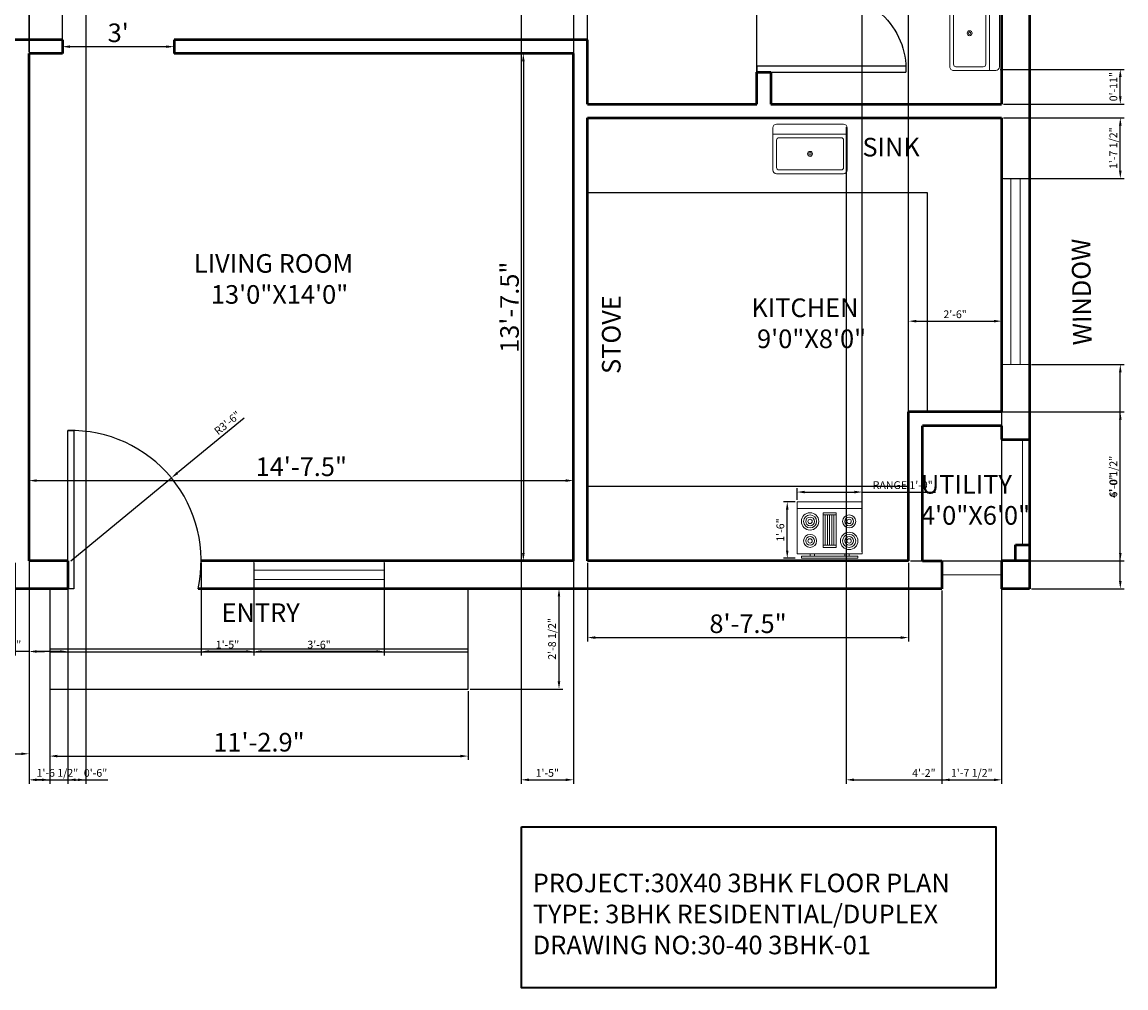
# Model space of a CAD drawing. Units: inches. Extents: x 259417 to 260009, y 246275 to 246915.
# Tile 2 of 4: x 259653 to 260009, y 246275 to 246587. Entities that reach past the tile are written whole.
import ezdxf

# ---------------------------------------------------------------- set-up
doc = ezdxf.new("R2010")
doc.units = ezdxf.units.IN
for name, color, linetype, lineweight in [('A-ANNO-DIMS', 2, 'Continuous', 18), ('A-ANNO-TEXT', 7, 'Continuous', 18), ('A-ANNO-TTLB', 7, 'Continuous', 35), ('A-AREA-IDEN', 7, 'Continuous', 25), ('A-DOOR', 3, 'Continuous', 25), ('A-EQPM', 9, 'Continuous', 18), ('A-FLOR-CASE', 9, 'Continuous', 25), ('A-FLOR-FIXT', 8, 'Continuous', 18), ('A-FLOR-STRS', 7, 'Continuous', 25), ('A-GLAZ', 4, 'Continuous', 18), ('A-WALL', 7, 'Continuous', 50)]:
    doc.layers.add(name, color=color, linetype=linetype, lineweight=lineweight)
doc.styles.get("Standard").update_dxf_attribs({"font": 'arial.ttf'})
doc.dimstyles.new('ISO-25', dxfattribs={"dimtxt": 2.5, "dimasz": 2.5, "dimexe": 1.25, "dimexo": 0.625, "dimtad": 1, "dimdec": 1, "dimlunit": 3, "dimtxsty": 'Standard', "dimcen": 2.5, "dimadec": 0, "dimazin": 0, "dimtfac": 1, "dimtdec": 1, "dimtmove": 0, "dimatfit": 3, "dimfxl": 1, "dimarcsym": 0})

# ---------------------------------------------------------------- blocks, each defined once
blk = doc.blocks.new('*D15')
at = {"layer": 'A-ANNO-DIMS', "color": 0, "lineweight": -2, "transparency": 16777216}
for p, q in [((259655.09, 246413.47), (259655.09, 246439.94)), ((259657.59, 246438.69), (259828.09, 246438.69)), ((259830.59, 246413.47), (259830.59, 246439.94))]:
    blk.add_line(p, q, dxfattribs=at)
at = {"layer": 'A-ANNO-DIMS', "color": 0, "transparency": 16777216}
for points in [[(259657.59, 246439.11), (259657.59, 246438.28), (259655.09, 246438.69)], [(259828.09, 246439.11), (259828.09, 246438.28), (259830.59, 246438.69)]]:
    blk.add_solid(points, dxfattribs=at)
at = {"layer": 'Defpoints', "color": 0, "transparency": 16777216}
for p in [(259830.59, 246438.69), (259655.09, 246412.84), (259830.59, 246412.84)]:
    blk.add_point(p, dxfattribs=at)
at = {"layer": 'A-ANNO-DIMS', "color": 0, "transparency": 16777216, "insert": (259742.84, 246442.38), "char_height": 6, "attachment_point": 5}
blk.add_mtext('14\'-7.5"', dxfattribs=at)
blk = doc.blocks.new('*D16')
at = {"layer": 'A-ANNO-DIMS', "color": 0, "lineweight": -2, "transparency": 16777216}
for p, q in [((259665.84, 246576.97), (259665.84, 246579.84)), ((259668.34, 246578.59), (259699.34, 246578.59)), ((259701.84, 246576.97), (259701.84, 246579.84))]:
    blk.add_line(p, q, dxfattribs=at)
at = {"layer": 'A-ANNO-DIMS', "color": 0, "transparency": 16777216}
for points in [[(259668.34, 246579.01), (259668.34, 246578.17), (259665.84, 246578.59)], [(259699.34, 246579.01), (259699.34, 246578.17), (259701.84, 246578.59)]]:
    blk.add_solid(points, dxfattribs=at)
at = {"layer": 'Defpoints', "color": 0, "transparency": 16777216}
for p in [(259701.84, 246578.59), (259665.84, 246576.34), (259701.84, 246576.34)]:
    blk.add_point(p, dxfattribs=at)
at = {"layer": 'A-ANNO-DIMS', "color": 0, "transparency": 16777216, "insert": (259683.84, 246582.28), "char_height": 6, "attachment_point": 5}
blk.add_mtext("3'", dxfattribs=at)
blk = doc.blocks.new('*D17')
at = {"layer": 'A-ANNO-DIMS', "color": 0, "lineweight": -2, "transparency": 16777216}
for p, q in [((259829.97, 246576.34), (259813.17, 246576.34)), ((259814.42, 246573.84), (259814.42, 246415.34)), ((259829.97, 246412.84), (259813.17, 246412.84))]:
    blk.add_line(p, q, dxfattribs=at)
at = {"layer": 'A-ANNO-DIMS', "color": 0, "transparency": 16777216}
for points in [[(259814, 246573.84), (259814.84, 246573.84), (259814.42, 246576.34)], [(259814, 246415.34), (259814.84, 246415.34), (259814.42, 246412.84)]]:
    blk.add_solid(points, dxfattribs=at)
at = {"layer": 'Defpoints', "color": 0, "transparency": 16777216}
for p in [(259830.59, 246576.34), (259814.42, 246412.84), (259830.59, 246412.84)]:
    blk.add_point(p, dxfattribs=at)
at = {"layer": 'A-ANNO-DIMS', "color": 0, "transparency": 16777216, "insert": (259810.73, 246494.59), "char_height": 6, "attachment_point": 5, "rotation": 90}
blk.add_mtext('13\'-7.5"', dxfattribs=at)
blk = doc.blocks.new('*D18')
at = {"layer": 'A-ANNO-DIMS', "color": 0, "lineweight": -2, "transparency": 16777216}
for p, q in [((259835.09, 246412.22), (259835.09, 246386.83)), ((259938.59, 246412.22), (259938.59, 246386.83)), ((259837.59, 246388.08), (259936.09, 246388.08))]:
    blk.add_line(p, q, dxfattribs=at)
at = {"layer": 'A-ANNO-DIMS', "color": 0, "transparency": 16777216}
for points in [[(259837.59, 246388.49), (259837.59, 246387.66), (259835.09, 246388.08)], [(259936.09, 246388.49), (259936.09, 246387.66), (259938.59, 246388.08)]]:
    blk.add_solid(points, dxfattribs=at)
at = {"layer": 'Defpoints', "color": 0, "transparency": 16777216}
for p in [(259835.09, 246412.84), (259938.59, 246412.84), (259938.59, 246388.08)]:
    blk.add_point(p, dxfattribs=at)
at = {"layer": 'A-ANNO-DIMS', "color": 0, "transparency": 16777216, "insert": (259886.84, 246391.77), "char_height": 6, "attachment_point": 5}
blk.add_mtext('8\'-7.5"', dxfattribs=at)
blk = doc.blocks.new('*D19')
at = {"layer": 'A-ANNO-DIMS', "color": 0, "lineweight": -2, "transparency": 16777216}
for p, q in [((259661.74, 246370.85), (259661.74, 246348.63)), ((259796.66, 246370.85), (259796.66, 246348.63)), ((259664.24, 246349.88), (259794.16, 246349.88))]:
    blk.add_line(p, q, dxfattribs=at)
at = {"layer": 'A-ANNO-DIMS', "color": 0, "transparency": 16777216}
for points in [[(259664.24, 246350.3), (259664.24, 246349.46), (259661.74, 246349.88)], [(259794.16, 246350.3), (259794.16, 246349.46), (259796.66, 246349.88)]]:
    blk.add_solid(points, dxfattribs=at)
at = {"layer": 'Defpoints', "color": 0, "transparency": 16777216}
for p in [(259661.74, 246371.48), (259796.66, 246371.48), (259796.66, 246349.88)]:
    blk.add_point(p, dxfattribs=at)
at = {"layer": 'A-ANNO-DIMS', "color": 0, "transparency": 16777216, "insert": (259729.2, 246353.57), "char_height": 6, "attachment_point": 5}
blk.add_mtext('11\'-2.9"', dxfattribs=at)
blk = doc.blocks.new('*D20')
at = {"layer": 'A-ANNO-DIMS', "color": 0, "lineweight": -2, "transparency": 16777216}
for p, q in [((259497.59, 246403.22), (259497.59, 246349.38)), ((259655.09, 246403.22), (259655.09, 246349.38)), ((259500.09, 246350.63), (259652.59, 246350.63))]:
    blk.add_line(p, q, dxfattribs=at)
at = {"layer": 'A-ANNO-DIMS', "color": 0, "transparency": 16777216}
for points in [[(259500.09, 246351.04), (259500.09, 246350.21), (259497.59, 246350.63)], [(259652.59, 246351.04), (259652.59, 246350.21), (259655.09, 246350.63)]]:
    blk.add_solid(points, dxfattribs=at)
at = {"layer": 'Defpoints', "color": 0, "transparency": 16777216}
for p in [(259497.59, 246403.84), (259655.09, 246403.84), (259655.09, 246350.63)]:
    blk.add_point(p, dxfattribs=at)
at = {"layer": 'A-ANNO-DIMS', "color": 0, "transparency": 16777216, "insert": (259576.34, 246354.32), "char_height": 6, "attachment_point": 5}
blk.add_mtext('13\'-1.5"', dxfattribs=at)
blk = doc.blocks.new('Range-Oven - 30 in top')
for p, q in [((0, -3), (30, -3)), ((12, -6), (18, -6)), ((13, -20), (13, -6)), ((14, -6), (14, -20)), ((15, -20), (15, -6)), ((16, -6), (16, -20)), ((17, -20), (17, -6)), ((18, -20), (12, -20)), ((6, -24), (6, -25)), ((8, -25), (8, -24)), ((22, -25), (22, -24)), ((24, -24), (24, -25))]:
    blk.add_line(p, q)
for points in [[(0, -24), (0, 0), (30, 0), (30, -24)], [(12, -21), (12, -5), (18, -5), (18, -21)], [(2, -26), (2, -25), (28, -25), (28, -26)]]:
    blk.add_lwpolyline(points, close=True)
for centre, radius in [((6, -9), 4), ((6, -9), 3), ((6, -9), 2), ((6, -9), 1), ((24, -9), 3), ((24, -9), 2), ((24, -9), 1), ((6, -18), 3), ((24, -18), 4), ((24, -18), 3), ((6, -18), 2), ((6, -18), 1), ((24, -18), 2), ((24, -18), 1)]:
    blk.add_circle(centre, radius)
blk = doc.blocks.new('Sink-single - 30 in top')
blk.add_line((-15, -3.999996), (15, -3.999996))
for points in [[(-13.5, 0), (13.5, 0)], [(-15, -18.499996), (-15, -1.5)], [(15, -1.5), (15, -18.499996)], [(-13.5, -17.499996), (-13.5, -6.499996)], [(-12.5, -5.499996), (12.5, -5.499996)], [(13.5, -6.499996), (13.5, -17.499996)], [(13.5, -19.999996), (-13.5, -19.999996)], [(12.5, -18.499996), (-12.5, -18.499996)]]:
    blk.add_lwpolyline(points)
for radius in [1, 0.5]:
    blk.add_circle((0, -11.999996), radius)
for centre, radius, start, end in [((-13.5, -1.5), 1.5, 90, 180), ((13.5, -1.5), 1.5, 0, 90), ((-12.5, -6.499996), 1, 90, 180), ((12.5, -6.499996), 1, 0, 90), ((-12.5, -17.499996), 1, 180, 270), ((12.5, -17.499996), 1, 270, 0), ((-13.5, -18.499996), 1.5, 180, 270), ((13.5, -18.499996), 1.5, 270, 0)]:
    blk.add_arc(centre, radius, start, end)
blk = doc.blocks.new('WIN-60x9')
for p, q in [((0, 9), (0, 0)), ((60, 9), (60, 0)), ((60, 6), (0, 6)), ((60, 3), (0, 3))]:
    blk.add_line(p, q)
blk = doc.blocks.new('DOOR-BATH-PAIRED-LEAF')
for p, q in [((0, 0), (48, 0)), ((0, -2), (0, 0)), ((48, -2), (0, -2)), ((48, -2), (48, 0))]:
    blk.add_line(p, q)
blk.add_arc((23.97, -1), 24.05, 263.254, 2.3829)
blk = doc.blocks.new('*D30')
at = {"layer": 'A-ANNO-DIMS', "color": 0, "lineweight": -2, "transparency": 16777216}
for p, q in [((259902.64, 246432.48), (259902.64, 246436.25)), ((259905.14, 246435), (259921.14, 246435)), ((259923.64, 246432.48), (259923.64, 246436.25)), ((259923.64, 246435), (259947.29, 246435))]:
    blk.add_line(p, q, dxfattribs=at)
at = {"layer": 'A-ANNO-DIMS', "color": 0, "transparency": 16777216}
for points in [[(259905.14, 246435.42), (259905.14, 246434.58), (259902.64, 246435)], [(259921.14, 246435.42), (259921.14, 246434.58), (259923.64, 246435)]]:
    blk.add_solid(points, dxfattribs=at)
at = {"layer": 'Defpoints', "color": 0, "transparency": 16777216}
for p in [(259923.64, 246435), (259902.64, 246431.85), (259923.64, 246431.85)]:
    blk.add_point(p, dxfattribs=at)
at = {"layer": 'A-ANNO-DIMS', "color": 0, "transparency": 16777216, "insert": (259936.71, 246436.92), "char_height": 2.5, "attachment_point": 5}
blk.add_mtext('RANGE 1\'-9"', dxfattribs=at)
blk = doc.blocks.new('*D31')
at = {"layer": 'A-ANNO-DIMS', "color": 0, "lineweight": -2, "transparency": 16777216}
for p, q in [((259902.01, 246431.85), (259898.24, 246431.85)), ((259899.49, 246416.15), (259899.49, 246429.35)), ((259902.01, 246413.65), (259898.24, 246413.65))]:
    blk.add_line(p, q, dxfattribs=at)
at = {"layer": 'A-ANNO-DIMS', "color": 0, "transparency": 16777216}
for points in [[(259899.07, 246429.35), (259899.9, 246429.35), (259899.49, 246431.85)], [(259899.07, 246416.15), (259899.9, 246416.15), (259899.49, 246413.65)]]:
    blk.add_solid(points, dxfattribs=at)
at = {"layer": 'Defpoints', "color": 0, "transparency": 16777216}
for p in [(259899.49, 246431.85), (259902.64, 246431.85), (259902.64, 246413.65)]:
    blk.add_point(p, dxfattribs=at)
at = {"layer": 'A-ANNO-DIMS', "color": 0, "transparency": 16777216, "insert": (259897.58, 246422.75), "char_height": 2.5, "attachment_point": 5, "rotation": 90}
blk.add_mtext('1\'-6"', dxfattribs=at)
blk = doc.blocks.new('*D37')
at = {"layer": 'A-ANNO-DIMS', "color": 0, "lineweight": -2, "transparency": 16777216}
for p, q in [((259978.22, 246476.12), (260008.09, 246476.12)), ((260006.84, 246406.34), (260006.84, 246473.62)), ((259978.22, 246403.84), (260008.09, 246403.84))]:
    blk.add_line(p, q, dxfattribs=at)
at = {"layer": 'A-ANNO-DIMS', "color": 0, "transparency": 16777216}
for points in [[(260006.42, 246473.62), (260007.26, 246473.62), (260006.84, 246476.12)], [(260006.42, 246406.34), (260007.26, 246406.34), (260006.84, 246403.84)]]:
    blk.add_solid(points, dxfattribs=at)
at = {"layer": 'Defpoints', "color": 0, "transparency": 16777216}
for p in [(259977.59, 246476.12), (260006.84, 246476.12), (259977.59, 246403.84)]:
    blk.add_point(p, dxfattribs=at)
at = {"layer": 'A-ANNO-DIMS', "color": 0, "transparency": 16777216, "insert": (260004.92, 246439.98), "char_height": 2.5, "attachment_point": 5, "rotation": 90}
blk.add_mtext('6\'-0 1/2"', dxfattribs=at)
blk = doc.blocks.new('*D40')
at = {"layer": 'A-ANNO-DIMS', "color": 0, "lineweight": -2, "transparency": 16777216}
for p, q in [((259727.57, 246412.22), (259727.57, 246382.34)), ((259769.57, 246412.22), (259769.57, 246382.34)), ((259767.07, 246383.59), (259730.07, 246383.59))]:
    blk.add_line(p, q, dxfattribs=at)
at = {"layer": 'A-ANNO-DIMS', "color": 0, "transparency": 16777216}
for points in [[(259730.07, 246384.01), (259730.07, 246383.17), (259727.57, 246383.59)], [(259767.07, 246384.01), (259767.07, 246383.17), (259769.57, 246383.59)]]:
    blk.add_solid(points, dxfattribs=at)
at = {"layer": 'Defpoints', "color": 0, "transparency": 16777216}
for p in [(259727.57, 246412.84), (259769.57, 246412.84), (259727.57, 246383.59)]:
    blk.add_point(p, dxfattribs=at)
at = {"layer": 'A-ANNO-DIMS', "color": 0, "transparency": 16777216, "insert": (259748.57, 246385.49), "char_height": 2.5, "attachment_point": 5}
blk.add_mtext('3\'-6"', dxfattribs=at)
blk = doc.blocks.new('*D41')
at = {"layer": 'A-ANNO-DIMS', "color": 0, "lineweight": -2, "transparency": 16777216}
for p, q in [((259797.28, 246403.84), (259827.16, 246403.84)), ((259825.91, 246401.34), (259825.91, 246373.98)), ((259797.28, 246371.48), (259827.16, 246371.48))]:
    blk.add_line(p, q, dxfattribs=at)
at = {"layer": 'A-ANNO-DIMS', "color": 0, "transparency": 16777216}
for points in [[(259825.49, 246401.34), (259826.32, 246401.34), (259825.91, 246403.84)], [(259825.49, 246373.98), (259826.32, 246373.98), (259825.91, 246371.48)]]:
    blk.add_solid(points, dxfattribs=at)
at = {"layer": 'Defpoints', "color": 0, "transparency": 16777216}
for p in [(259796.66, 246403.84), (259796.66, 246371.48), (259825.91, 246371.48)]:
    blk.add_point(p, dxfattribs=at)
at = {"layer": 'A-ANNO-DIMS', "color": 0, "transparency": 16777216, "insert": (259823.99, 246387.66), "char_height": 2.5, "attachment_point": 5, "rotation": 90}
blk.add_mtext('2\'-8 1/2"', dxfattribs=at)
blk = doc.blocks.new('*D43')
at = {"layer": 'A-ANNO-DIMS', "color": 0, "lineweight": -2, "transparency": 16777216}
for p, q in [((259650.59, 246412.22), (259650.59, 246382.34)), ((259655.09, 246412.22), (259655.09, 246382.34)), ((259648.09, 246383.59), (259631.87, 246383.59)), ((259655.09, 246383.59), (259650.59, 246383.59)), ((259657.59, 246383.59), (259660.09, 246383.59))]:
    blk.add_line(p, q, dxfattribs=at)
at = {"layer": 'A-ANNO-DIMS', "color": 0, "transparency": 16777216}
for points in [[(259648.09, 246384.01), (259648.09, 246383.17), (259650.59, 246383.59)], [(259657.59, 246384.01), (259657.59, 246383.17), (259655.09, 246383.59)]]:
    blk.add_solid(points, dxfattribs=at)
at = {"layer": 'Defpoints', "color": 0, "transparency": 16777216}
for p in [(259650.59, 246412.84), (259655.09, 246412.84), (259650.59, 246383.59)]:
    blk.add_point(p, dxfattribs=at)
at = {"layer": 'A-ANNO-DIMS', "color": 0, "transparency": 16777216, "insert": (259638.73, 246385.51), "char_height": 2.5, "attachment_point": 5}
blk.add_mtext('0\'-4 1/2"', dxfattribs=at)
blk = doc.blocks.new('*D44')
at = {"layer": 'A-ANNO-DIMS', "color": 0, "lineweight": -2, "transparency": 16777216}
for p, q in [((259655.09, 246412.22), (259655.09, 246382.34)), ((259667.57, 246412.22), (259667.57, 246382.34)), ((259655.09, 246383.59), (259639.11, 246383.59)), ((259665.07, 246383.59), (259657.59, 246383.59))]:
    blk.add_line(p, q, dxfattribs=at)
at = {"layer": 'A-ANNO-DIMS', "color": 0, "transparency": 16777216}
for points in [[(259657.59, 246384.01), (259657.59, 246383.17), (259655.09, 246383.59)], [(259665.07, 246384.01), (259665.07, 246383.17), (259667.57, 246383.59)]]:
    blk.add_solid(points, dxfattribs=at)
at = {"layer": 'Defpoints', "color": 0, "transparency": 16777216}
for p in [(259655.09, 246412.84), (259667.57, 246412.84), (259655.09, 246383.59)]:
    blk.add_point(p, dxfattribs=at)
at = {"layer": 'A-ANNO-DIMS', "color": 0, "transparency": 16777216, "insert": (259645.85, 246385.51), "char_height": 2.5, "attachment_point": 5}
blk.add_mtext('1\'-0 1/2"', dxfattribs=at)
blk = doc.blocks.new('*D45')
at = {"layer": 'A-ANNO-DIMS', "color": 0, "lineweight": -2, "transparency": 16777216}
for p, q in [((259710.55, 246412.22), (259710.55, 246382.34)), ((259727.57, 246412.22), (259727.57, 246382.34)), ((259725.07, 246383.59), (259713.05, 246383.59))]:
    blk.add_line(p, q, dxfattribs=at)
at = {"layer": 'A-ANNO-DIMS', "color": 0, "transparency": 16777216}
for points in [[(259713.05, 246384.01), (259713.05, 246383.17), (259710.55, 246383.59)], [(259725.07, 246384.01), (259725.07, 246383.17), (259727.57, 246383.59)]]:
    blk.add_solid(points, dxfattribs=at)
at = {"layer": 'Defpoints', "color": 0, "transparency": 16777216}
for p in [(259710.55, 246412.84), (259727.57, 246412.84), (259710.55, 246383.59)]:
    blk.add_point(p, dxfattribs=at)
at = {"layer": 'A-ANNO-DIMS', "color": 0, "transparency": 16777216, "insert": (259719.06, 246385.49), "char_height": 2.5, "attachment_point": 5}
blk.add_mtext('1\'-5"', dxfattribs=at)
blk = doc.blocks.new('*D46')
at = {"layer": 'A-ANNO-DIMS', "color": 0, "lineweight": -2, "transparency": 16777216}
for p, q in [((259938.59, 246461.47), (259938.59, 246491.34)), ((259968.59, 246461.47), (259968.59, 246491.34)), ((259941.09, 246490.09), (259966.09, 246490.09))]:
    blk.add_line(p, q, dxfattribs=at)
at = {"layer": 'A-ANNO-DIMS', "color": 0, "transparency": 16777216}
for points in [[(259941.09, 246490.51), (259941.09, 246489.67), (259938.59, 246490.09)], [(259966.09, 246490.51), (259966.09, 246489.67), (259968.59, 246490.09)]]:
    blk.add_solid(points, dxfattribs=at)
at = {"layer": 'Defpoints', "color": 0, "transparency": 16777216}
for p in [(259968.59, 246490.09), (259938.59, 246460.84), (259968.59, 246460.84)]:
    blk.add_point(p, dxfattribs=at)
at = {"layer": 'A-ANNO-DIMS', "color": 0, "transparency": 16777216, "insert": (259953.59, 246491.99), "char_height": 2.5, "attachment_point": 5}
blk.add_mtext('2\'-6"', dxfattribs=at)
blk = doc.blocks.new('*D47')
at = {"layer": 'A-ANNO-DIMS', "color": 0, "lineweight": -2, "transparency": 16777216}
for p, q in [((259939.22, 246460.84), (260008.09, 246460.84)), ((260006.84, 246415.34), (260006.84, 246458.34)), ((259939.22, 246412.84), (260008.09, 246412.84))]:
    blk.add_line(p, q, dxfattribs=at)
at = {"layer": 'A-ANNO-DIMS', "color": 0, "transparency": 16777216}
for points in [[(260006.42, 246458.34), (260007.26, 246458.34), (260006.84, 246460.84)], [(260006.42, 246415.34), (260007.26, 246415.34), (260006.84, 246412.84)]]:
    blk.add_solid(points, dxfattribs=at)
at = {"layer": 'Defpoints', "color": 0, "transparency": 16777216}
for p in [(259938.59, 246460.84), (260006.84, 246460.84), (259938.59, 246412.84)]:
    blk.add_point(p, dxfattribs=at)
at = {"layer": 'A-ANNO-DIMS', "color": 0, "transparency": 16777216, "insert": (260004.94, 246436.84), "char_height": 2.5, "attachment_point": 5, "rotation": 90}
blk.add_mtext('4\'-0"', dxfattribs=at)
blk = doc.blocks.new('*D48')
at = {"layer": 'A-ANNO-DIMS', "color": 0, "lineweight": -2, "transparency": 16777216}
for p, q in [((259969.22, 246555.6), (260008.09, 246555.6)), ((260006.84, 246538.62), (260006.84, 246553.1)), ((259969.22, 246536.12), (260008.09, 246536.12))]:
    blk.add_line(p, q, dxfattribs=at)
at = {"layer": 'A-ANNO-DIMS', "color": 0, "transparency": 16777216}
for points in [[(260006.42, 246553.1), (260007.26, 246553.1), (260006.84, 246555.6)], [(260006.42, 246538.62), (260007.26, 246538.62), (260006.84, 246536.12)]]:
    blk.add_solid(points, dxfattribs=at)
at = {"layer": 'Defpoints', "color": 0, "transparency": 16777216}
for p in [(259968.59, 246555.6), (260006.84, 246555.6), (259968.59, 246536.12)]:
    blk.add_point(p, dxfattribs=at)
at = {"layer": 'A-ANNO-DIMS', "color": 0, "transparency": 16777216, "insert": (260004.92, 246545.86), "char_height": 2.5, "attachment_point": 5, "rotation": 90}
blk.add_mtext('1\'-7 1/2"', dxfattribs=at)
blk = doc.blocks.new('*D49')
at = {"layer": 'A-ANNO-DIMS', "color": 0, "lineweight": -2, "transparency": 16777216}
for p, q in [((259835.09, 246560.72), (259835.09, 246590.6)), ((259837.59, 246589.35), (259887.21, 246589.35)), ((259889.71, 246560.72), (259889.71, 246590.6))]:
    blk.add_line(p, q, dxfattribs=at)
at = {"layer": 'A-ANNO-DIMS', "color": 0, "transparency": 16777216}
for points in [[(259837.59, 246589.77), (259837.59, 246588.93), (259835.09, 246589.35)], [(259887.21, 246589.77), (259887.21, 246588.93), (259889.71, 246589.35)]]:
    blk.add_solid(points, dxfattribs=at)
at = {"layer": 'Defpoints', "color": 0, "transparency": 16777216}
for p in [(259889.71, 246589.35), (259835.09, 246560.1), (259889.71, 246560.1)]:
    blk.add_point(p, dxfattribs=at)
at = {"layer": 'A-ANNO-DIMS', "color": 0, "transparency": 16777216, "insert": (259862.4, 246591.27), "char_height": 2.5, "attachment_point": 5}
blk.add_mtext('4\'-6 1/2"', dxfattribs=at)
blk = doc.blocks.new('*D53')
at = {"layer": 'A-ANNO-DIMS', "color": 0, "lineweight": -2, "transparency": 16777216}
for p, q in [((259655.09, 246576.97), (259655.09, 246606.84)), ((259657.59, 246605.59), (259663.34, 246605.59)), ((259665.84, 246576.97), (259665.84, 246606.84)), ((259665.84, 246605.59), (259684, 246605.59))]:
    blk.add_line(p, q, dxfattribs=at)
at = {"layer": 'A-ANNO-DIMS', "color": 0, "transparency": 16777216}
for points in [[(259657.59, 246606.01), (259657.59, 246605.17), (259655.09, 246605.59)], [(259663.34, 246606.01), (259663.34, 246605.17), (259665.84, 246605.59)]]:
    blk.add_solid(points, dxfattribs=at)
at = {"layer": 'Defpoints', "color": 0, "transparency": 16777216}
for p in [(259665.84, 246605.59), (259655.09, 246576.34), (259665.84, 246576.34)]:
    blk.add_point(p, dxfattribs=at)
at = {"layer": 'A-ANNO-DIMS', "color": 0, "transparency": 16777216, "insert": (259676.17, 246607.51), "char_height": 2.5, "attachment_point": 5}
blk.add_mtext('0\'-10 1/2"', dxfattribs=at)
blk = doc.blocks.new('*D54')
at = {"layer": 'A-ANNO-DIMS', "color": 0, "lineweight": -2, "transparency": 16777216}
for p, q in [((259949.33, 246403.22), (259949.33, 246340.98)), ((259968.59, 246403.22), (259968.59, 246340.98)), ((259951.83, 246342.23), (259966.09, 246342.23))]:
    blk.add_line(p, q, dxfattribs=at)
at = {"layer": 'A-ANNO-DIMS', "color": 0, "transparency": 16777216}
for points in [[(259951.83, 246342.64), (259951.83, 246341.81), (259949.33, 246342.23)], [(259966.09, 246342.64), (259966.09, 246341.81), (259968.59, 246342.23)]]:
    blk.add_solid(points, dxfattribs=at)
at = {"layer": 'Defpoints', "color": 0, "transparency": 16777216}
for p in [(259949.33, 246403.84), (259968.59, 246403.84), (259968.59, 246342.23)]:
    blk.add_point(p, dxfattribs=at)
at = {"layer": 'A-ANNO-DIMS', "color": 0, "transparency": 16777216, "insert": (259958.96, 246344.15), "char_height": 2.5, "attachment_point": 5}
blk.add_mtext('1\'-7 1/2"', dxfattribs=at)
blk = doc.blocks.new('*D56')
at = {"layer": 'A-ANNO-DIMS', "color": 0, "lineweight": -2, "transparency": 16777216}
for p, q in [((259968.15, 246571.28), (260008.09, 246571.28)), ((260006.84, 246562.6), (260006.84, 246568.78)), ((259969.22, 246560.1), (260008.09, 246560.1))]:
    blk.add_line(p, q, dxfattribs=at)
at = {"layer": 'A-ANNO-DIMS', "color": 0, "transparency": 16777216}
for points in [[(260006.42, 246568.78), (260007.26, 246568.78), (260006.84, 246571.28)], [(260006.42, 246562.6), (260007.26, 246562.6), (260006.84, 246560.1)]]:
    blk.add_solid(points, dxfattribs=at)
at = {"layer": 'Defpoints', "color": 0, "transparency": 16777216}
for p in [(259967.52, 246571.28), (260006.84, 246571.28), (259968.59, 246560.1)]:
    blk.add_point(p, dxfattribs=at)
at = {"layer": 'A-ANNO-DIMS', "color": 0, "transparency": 16777216, "insert": (260004.94, 246565.69), "char_height": 2.5, "attachment_point": 5, "rotation": 90}
blk.add_mtext('0\'-11"', dxfattribs=at)
blk = doc.blocks.new('*D58')
at = {"layer": 'A-ANNO-DIMS', "color": 0, "lineweight": -2, "transparency": 16777216}
for p, q in [((259918.48, 246552.66), (259918.48, 246340.98)), ((259968.59, 246554.97), (259968.59, 246340.98)), ((259920.98, 246342.23), (259966.09, 246342.23))]:
    blk.add_line(p, q, dxfattribs=at)
at = {"layer": 'A-ANNO-DIMS', "color": 0, "transparency": 16777216}
for points in [[(259920.98, 246342.64), (259920.98, 246341.81), (259918.48, 246342.23)], [(259966.09, 246342.64), (259966.09, 246341.81), (259968.59, 246342.23)]]:
    blk.add_solid(points, dxfattribs=at)
at = {"layer": 'Defpoints', "color": 0, "transparency": 16777216}
for p in [(259968.59, 246555.6), (259918.48, 246553.28), (259968.59, 246342.23)]:
    blk.add_point(p, dxfattribs=at)
at = {"layer": 'A-ANNO-DIMS', "color": 0, "transparency": 16777216, "insert": (259943.53, 246344.11), "char_height": 2.5, "attachment_point": 5}
blk.add_mtext('4\'-2"', dxfattribs=at)
blk = doc.blocks.new('*D59')
at = {"layer": 'A-ANNO-DIMS', "color": 0, "lineweight": -2, "transparency": 16777216}
for p, q in [((259923.64, 246415.68), (259923.64, 246794.34)), ((259938.59, 246413.47), (259938.59, 246794.34)), ((259926.14, 246793.09), (259936.09, 246793.09))]:
    blk.add_line(p, q, dxfattribs=at)
at = {"layer": 'A-ANNO-DIMS', "color": 0, "transparency": 16777216}
for points in [[(259926.14, 246793.51), (259926.14, 246792.67), (259923.64, 246793.09)], [(259936.09, 246793.51), (259936.09, 246792.67), (259938.59, 246793.09)]]:
    blk.add_solid(points, dxfattribs=at)
at = {"layer": 'Defpoints', "color": 0, "transparency": 16777216}
for p in [(259938.59, 246793.09), (259923.64, 246415.05), (259938.59, 246412.84)]:
    blk.add_point(p, dxfattribs=at)
at = {"layer": 'A-ANNO-DIMS', "color": 0, "transparency": 16777216, "insert": (259931.11, 246794.99), "char_height": 2.5, "attachment_point": 5}
blk.add_mtext('1\'-3"', dxfattribs=at)
blk = doc.blocks.new('*D62')
at = {"layer": 'A-ANNO-DIMS', "color": 0, "lineweight": -2, "transparency": 16777216}
for p, q in [((259655.09, 246714.26), (259655.09, 246340.98)), ((259673.35, 246711.84), (259673.35, 246340.98)), ((259657.59, 246342.23), (259670.85, 246342.23))]:
    blk.add_line(p, q, dxfattribs=at)
at = {"layer": 'A-ANNO-DIMS', "color": 0, "transparency": 16777216}
for points in [[(259657.59, 246342.64), (259657.59, 246341.81), (259655.09, 246342.23)], [(259670.85, 246342.64), (259670.85, 246341.81), (259673.35, 246342.23)]]:
    blk.add_solid(points, dxfattribs=at)
at = {"layer": 'Defpoints', "color": 0, "transparency": 16777216}
for p in [(259655.09, 246714.89), (259673.35, 246712.46), (259673.35, 246342.23)]:
    blk.add_point(p, dxfattribs=at)
at = {"layer": 'A-ANNO-DIMS', "color": 0, "transparency": 16777216, "insert": (259664.22, 246344.15), "char_height": 2.5, "attachment_point": 5}
blk.add_mtext('1\'-6 1/2"', dxfattribs=at)
blk = doc.blocks.new('*D63')
at = {"layer": 'A-ANNO-DIMS', "color": 0, "lineweight": -2, "transparency": 16777216}
for p, q in [((259830.59, 246714.26), (259830.59, 246340.98)), ((259813.7, 246710.38), (259813.7, 246340.98)), ((259816.2, 246342.23), (259828.09, 246342.23))]:
    blk.add_line(p, q, dxfattribs=at)
at = {"layer": 'A-ANNO-DIMS', "color": 0, "transparency": 16777216}
for points in [[(259816.2, 246342.64), (259816.2, 246341.81), (259813.7, 246342.23)], [(259828.09, 246342.64), (259828.09, 246341.81), (259830.59, 246342.23)]]:
    blk.add_solid(points, dxfattribs=at)
at = {"layer": 'Defpoints', "color": 0, "transparency": 16777216}
for p in [(259830.59, 246714.89), (259813.7, 246711.01), (259830.59, 246342.23)]:
    blk.add_point(p, dxfattribs=at)
at = {"layer": 'A-ANNO-DIMS', "color": 0, "transparency": 16777216, "insert": (259822.14, 246344.13), "char_height": 2.5, "attachment_point": 5}
blk.add_mtext('1\'-5"', dxfattribs=at)
blk = doc.blocks.new('*D64')
at = {"layer": 'A-ANNO-DIMS', "color": 0, "lineweight": -2, "transparency": 16777216}
for p, q in [((259661.74, 246403.22), (259661.74, 246340.98)), ((259667.57, 246403.22), (259667.57, 246340.98)), ((259659.24, 246342.23), (259656.74, 246342.23)), ((259661.74, 246342.23), (259667.57, 246342.23)), ((259670.07, 246342.23), (259680.46, 246342.23))]:
    blk.add_line(p, q, dxfattribs=at)
at = {"layer": 'A-ANNO-DIMS', "color": 0, "transparency": 16777216}
for points in [[(259659.24, 246342.64), (259659.24, 246341.81), (259661.74, 246342.23)], [(259670.07, 246342.64), (259670.07, 246341.81), (259667.57, 246342.23)]]:
    blk.add_solid(points, dxfattribs=at)
at = {"layer": 'Defpoints', "color": 0, "transparency": 16777216}
for p in [(259661.74, 246403.84), (259667.57, 246403.84), (259667.57, 246342.23)]:
    blk.add_point(p, dxfattribs=at)
at = {"layer": 'A-ANNO-DIMS', "color": 0, "transparency": 16777216, "insert": (259676.52, 246344.13), "char_height": 2.5, "attachment_point": 5}
blk.add_mtext('0\'-6"', dxfattribs=at)
blk = doc.blocks.new('*D65')
at = {"layer": 'A-ANNO-DIMS', "color": 0, "lineweight": -2, "transparency": 16777216}
for p, q in [((259724.39, 246458.84), (259702.9, 246441.15)), ((259668.57, 246412.87), (259700.97, 246439.56))]:
    blk.add_line(p, q, dxfattribs=at)
at = {"layer": 'A-ANNO-DIMS', "color": 0, "transparency": 16777216}
blk.add_solid([(259702.64, 246441.47), (259703.17, 246440.83), (259700.97, 246439.56)], dxfattribs=at)
at = {"layer": 'Defpoints', "color": 0, "transparency": 16777216}
for p in [(259700.97, 246439.56), (259668.57, 246412.87)]:
    blk.add_point(p, dxfattribs=at)
at = {"layer": 'A-ANNO-DIMS', "color": 0, "transparency": 16777216, "insert": (259719.21, 246457.04), "char_height": 2.5, "attachment_point": 5, "rotation": 39.4728}
blk.add_mtext('R3\'-6"', dxfattribs=at)

msp = doc.modelspace()

# ---------------------------------------------------------------- linework, layer by layer
at = {"layer": 'A-ANNO-TTLB'}
msp.add_lwpolyline([(259813.79, 246327.11), (259966.71, 246327.11), (259966.71, 246275.14), (259813.79, 246275.14)], close=True, dxfattribs=at)
at = {"layer": 'A-DOOR'}
for p, q in [((259667.57, 246412.84), (259667.57, 246454.84)), ((259667.57, 246454.84), (259669.57, 246454.84)), ((259669.57, 246454.84), (259669.57, 246403.84)), ((259669.57, 246403.84), (259667.57, 246403.84))]:
    msp.add_line(p, q, dxfattribs=at)
msp.add_arc((259668.57, 246412.87), 41.98, 347.58, 91.3649, dxfattribs=at)
at = {"layer": 'A-FLOR-CASE'}
for p, q in [((259835.09, 246531.6), (259944.59, 246531.6)), ((259944.59, 246531.6), (259944.59, 246460.84)), ((259938.59, 246436.84), (259835.09, 246436.84))]:
    msp.add_line(p, q, dxfattribs=at)
at = {"layer": 'A-FLOR-STRS'}
for p, q in [((259661.74, 246403.84), (259661.74, 246371.48)), ((259796.66, 246371.48), (259796.66, 246403.84)), ((259661.74, 246384.48), (259796.66, 246384.48)), ((259661.74, 246383.48), (259796.66, 246383.48)), ((259661.74, 246371.48), (259796.66, 246371.48))]:
    msp.add_line(p, q, dxfattribs=at)
at = {"layer": 'A-GLAZ'}
for p, q in [((259975.34, 246418), (259975.34, 246451.96)), ((259727.57, 246412.84), (259727.57, 246403.84)), ((259769.57, 246409.84), (259727.57, 246409.84)), ((259769.57, 246412.84), (259769.57, 246403.84)), ((259769.57, 246406.84), (259727.57, 246406.84)), ((259949.33, 246408.34), (259968.59, 246408.34))]:
    msp.add_line(p, q, dxfattribs=at)
at = {"layer": 'A-WALL'}
for p, q in [((259977.59, 246763.84), (259977.59, 246403.84)), ((259968.59, 246630.34), (259968.59, 246560.1)), ((259665.84, 246580.84), (259644.83, 246580.84)), ((259665.84, 246580.84), (259665.84, 246576.34)), ((259835.09, 246580.84), (259701.84, 246580.84)), ((259701.84, 246580.84), (259701.84, 246576.34)), ((259835.09, 246560.1), (259835.09, 246580.84)), ((259655.09, 246412.84), (259655.09, 246576.34)), ((259665.84, 246576.34), (259655.09, 246576.34)), ((259830.59, 246576.34), (259701.84, 246576.34)), ((259830.59, 246412.84), (259830.59, 246576.34)), ((259889.71, 246560.1), (259889.71, 246570.33)), ((259889.71, 246570.33), (259894.21, 246570.33)), ((259894.21, 246570.33), (259894.21, 246560.1)), ((259835.09, 246560.1), (259889.71, 246560.1)), ((259894.21, 246560.1), (259968.59, 246560.1)), ((259835.09, 246412.84), (259835.09, 246555.6)), ((259835.09, 246555.6), (259968.59, 246555.6)), ((259968.59, 246555.6), (259968.59, 246460.84)), ((259938.59, 246412.84), (259938.59, 246460.84)), ((259968.59, 246460.84), (259938.59, 246460.84)), ((259943.09, 246412.84), (259943.09, 246456.34)), ((259968.59, 246456.34), (259943.09, 246456.34)), ((259968.59, 246456.34), (259968.59, 246451.96)), ((259968.59, 246451.96), (259977.59, 246451.96)), ((259973.09, 246412.84), (259973.09, 246418)), ((259973.09, 246418), (259977.59, 246418)), ((259667.57, 246412.84), (259655.09, 246412.84)), ((259667.57, 246412.84), (259667.57, 246403.84)), ((259830.59, 246412.84), (259710.55, 246412.84)), ((259938.59, 246412.84), (259835.09, 246412.84)), ((259943.09, 246412.84), (259949.33, 246412.84)), ((259949.33, 246412.84), (259949.33, 246403.84)), ((259977.59, 246412.84), (259968.59, 246412.84)), ((259968.59, 246412.84), (259968.59, 246403.84)), ((259667.57, 246403.84), (259497.59, 246403.84)), ((259943.09, 246403.84), (259709.57, 246403.84)), ((259949.33, 246403.84), (259943.09, 246403.84)), ((259977.59, 246403.84), (259968.59, 246403.84))]:
    msp.add_line(p, q, dxfattribs=at)

# ---------------------------------------------------------------- block references
at = {"layer": 'A-DOOR', "extrusion": (0, 0, -1), "zscale": -1, "rotation": 180}
msp.add_blockref('DOOR-BATH-PAIRED-LEAF', (-259889.71, 246570.33), dxfattribs=at)
at = {"layer": 'A-EQPM', "xscale": 0.7, "yscale": 0.7, "zscale": 0.7}
msp.add_blockref('Range-Oven - 30 in top', (259902.64, 246431.85), dxfattribs=at)
at = {"layer": 'A-FLOR-FIXT', "xscale": 0.8, "yscale": 0.8, "zscale": 0.8, "rotation": 270}
msp.add_blockref('Sink-single - 30 in top', (259967.87, 246582.92), dxfattribs=at)
at = {"layer": 'A-FLOR-FIXT', "xscale": 0.8, "yscale": 0.8, "zscale": 0.8}
msp.add_blockref('Sink-single - 30 in top', (259906.83, 246553.63), dxfattribs=at)
at = {"layer": 'A-GLAZ', "rotation": 89.99999999994564}
msp.add_blockref('WIN-60x9', (259977.59, 246476.12), dxfattribs=at)

# ---------------------------------------------------------------- texts
at = {"layer": 'A-ANNO-TEXT', "insert": (259921.88, 246549.2), "char_height": 6, "attachment_point": 1}
msp.add_mtext_dynamic_manual_height_columns(' SINK', width=60.426, gutter_width=12.5, heights=[18.16], dxfattribs=at)
at = {"layer": 'A-ANNO-TEXT', "char_height": 6, "attachment_point": 1}
for s, insert, rotation in [('     WINDOW', (259991.73, 246473.11), 90.8169), (' STOVE', (259839.76, 246471.24), 90)]:
    msp.add_mtext_dynamic_manual_height_columns(s, width=60.426, gutter_width=12.5, heights=[18.16], dxfattribs=dict(at, insert=insert, rotation=rotation))
at = {"layer": 'A-ANNO-TTLB', "insert": (259813.79, 246311.98), "char_height": 6, "attachment_point": 1}
msp.add_mtext_dynamic_manual_height_columns('  PROJECT:30X40 3BHK FLOOR PLAN\\P  TYPE: 3BHK RESIDENTIAL/DUPLEX\\P  DRAWING NO:30-40 3BHK-01', width=174.7302, gutter_width=12.5, heights=[85.05], dxfattribs=at)
at = {"layer": 'A-AREA-IDEN', "char_height": 6, "attachment_point": 1}
for s, width, heights, insert in [('   LIVING ROOM\\P      13\'0"X14\'0"', 87.6317, [39.22], (259702.71, 246511.71)), (' KITCHEN\\P  9\'0"X8\'0"', 72.4491, [28.3], (259886.08, 246497.41)), (' UTILITY\\P 4\'0"X6\'0"', 60.426, [18.16], (259940.76, 246440.48)), ('     ENTRY', 60.426, [18.16], (259707.98, 246399.12))]:
    msp.add_mtext_dynamic_manual_height_columns(s, width=width, gutter_width=12.5, heights=heights, dxfattribs=dict(at, insert=insert))

# ---------------------------------------------------------------- dimensions: what is measured, and where the dimension line sits
at = {"layer": 'A-ANNO-DIMS'}
for base, p1, p2, override, picture, middle in [((259938.5916, 246793.0906), (259923.635, 246415.0514), (259938.5916, 246412.8406), {"dimdec": 1, "dimlfac": 1, "dimrnd": 0, "dimzin": 1, "dimdsep": 46, "dimlunit": 4, "dimfrac": 2}, '*D59', (259931.1133, 246794.9929)), ((259673.35, 246342.23), (259655.09, 246714.89), (259673.35, 246712.46), {"dimdec": 1, "dimlfac": 1, "dimrnd": 0, "dimzin": 1, "dimdsep": 46, "dimlunit": 4, "dimfrac": 2}, '*D62', (259664.22, 246344.15)), ((259830.59, 246342.23), (259813.7, 246711.01), (259830.59, 246714.89), {"dimdec": 1, "dimlfac": 1, "dimrnd": 0, "dimzin": 1, "dimdsep": 46, "dimlunit": 4, "dimfrac": 2}, '*D63', (259822.14, 246344.13)), ((259889.71, 246589.35), (259835.09, 246560.1), (259889.71, 246560.1), {"dimdec": 1, "dimlfac": 1, "dimrnd": 0, "dimzin": 1, "dimdsep": 46, "dimlunit": 4, "dimfrac": 2}, '*D49', (259862.4, 246591.27)), ((259701.84, 246578.59), (259665.84, 246576.34), (259701.84, 246576.34), {"dimtxt": 6, "dimclrd": 0, "dimclre": 0, "dimclrt": 0}, '*D16', (259683.84, 246582.28)), ((259968.59, 246342.23), (259918.48, 246553.28), (259968.59, 246555.6), {"dimdec": 1, "dimlfac": 1, "dimrnd": 0, "dimzin": 1, "dimdsep": 46, "dimlunit": 4, "dimfrac": 2}, '*D58', (259943.53, 246344.11)), ((259968.59, 246490.09), (259938.59, 246460.84), (259968.59, 246460.84), {"dimdec": 1, "dimlfac": 1, "dimrnd": 0, "dimzin": 1, "dimdsep": 46, "dimlunit": 4, "dimfrac": 2}, '*D46', (259953.59, 246491.99)), ((259830.59, 246438.69), (259655.09, 246412.84), (259830.59, 246412.84), {"dimtxt": 6, "dimclrd": 0, "dimclre": 0, "dimclrt": 0}, '*D15', (259742.84, 246442.38)), ((259938.59, 246388.08), (259835.09, 246412.84), (259938.59, 246412.84), {"dimtxt": 6, "dimclrd": 0, "dimclre": 0, "dimclrt": 0}, '*D18', (259886.84, 246391.77)), ((259655.09, 246350.63), (259497.59, 246403.84), (259655.09, 246403.84), {"dimtxt": 6, "dimclrd": 0, "dimclre": 0, "dimclrt": 0}, '*D20', (259576.34, 246354.32)), ((259667.57, 246342.23), (259661.74, 246403.84), (259667.57, 246403.84), {"dimdec": 1, "dimlfac": 1, "dimrnd": 0, "dimzin": 1, "dimdsep": 46, "dimlunit": 4, "dimfrac": 2}, '*D64', (259676.52, 246344.13)), ((259968.59, 246342.23), (259949.33, 246403.84), (259968.59, 246403.84), {"dimdec": 1, "dimlfac": 1, "dimrnd": 0, "dimzin": 1, "dimdsep": 46, "dimlunit": 4, "dimfrac": 2}, '*D54', (259958.96, 246344.15)), ((259796.66, 246349.88), (259661.74, 246371.48), (259796.66, 246371.48), {"dimtxt": 6, "dimclrd": 0, "dimclre": 0, "dimclrt": 0}, '*D19', (259729.2, 246353.57))]:
    dim = msp.add_linear_dim(base=base, p1=p1, p2=p2, dimstyle='ISO-25', override=override, dxfattribs=at)
    dim.commit()
    dim.dimension.update_dxf_attribs({"geometry": picture, "text_midpoint": middle})
for base, p1, p2, angle, override, picture, middle in [((259665.8375, 246605.5906), (259655.0916, 246576.3406), (259665.8375, 246576.3406), 0, {"dimdec": 1, "dimlfac": 1, "dimrnd": 0, "dimzin": 1, "dimdsep": 46, "dimlunit": 4, "dimfrac": 2}, '*D53', (259676.1692, 246607.5082)), ((259814.42, 246412.84), (259830.59, 246576.34), (259830.59, 246412.84), 90, {"dimtxt": 6, "dimclrd": 0, "dimclre": 0, "dimclrt": 0}, '*D17', (259810.73, 246494.59)), ((260006.84, 246571.28), (259968.59, 246560.1), (259967.52, 246571.28), 90, {"dimdec": 1, "dimlfac": 1, "dimrnd": 0, "dimzin": 1, "dimdsep": 46, "dimlunit": 4, "dimfrac": 2}, '*D56', (260004.94, 246565.69)), ((260006.84, 246555.6), (259968.59, 246536.12), (259968.59, 246555.6), 90, {"dimdec": 1, "dimlfac": 1, "dimrnd": 0, "dimzin": 1, "dimdsep": 46, "dimlunit": 4, "dimfrac": 2}, '*D48', (260004.92, 246545.86)), ((260006.84, 246476.12), (259977.59, 246403.84), (259977.59, 246476.12), 90, {"dimdec": 1, "dimlfac": 1, "dimrnd": 0, "dimzin": 1, "dimdsep": 46, "dimlunit": 4, "dimfrac": 2}, '*D37', (260004.92, 246439.98)), ((260006.84, 246460.84), (259938.59, 246412.84), (259938.59, 246460.84), 90, {"dimdec": 1, "dimlfac": 1, "dimrnd": 0, "dimzin": 1, "dimdsep": 46, "dimlunit": 4, "dimfrac": 2}, '*D47', (260004.94, 246436.84)), ((259899.49, 246431.85), (259902.64, 246413.65), (259902.64, 246431.85), 90, {"dimdec": 1, "dimlfac": 1, "dimrnd": 0, "dimzin": 1, "dimdsep": 46, "dimlunit": 4, "dimfrac": 2}, '*D31', (259897.58, 246422.75)), ((259650.59, 246383.59), (259655.09, 246412.84), (259650.59, 246412.84), 180, {"dimdec": 1, "dimlfac": 1, "dimrnd": 0, "dimzin": 1, "dimdsep": 46, "dimlunit": 4, "dimfrac": 2}, '*D43', (259638.73, 246385.51)), ((259655.09, 246383.59), (259667.57, 246412.84), (259655.09, 246412.84), 180, {"dimdec": 1, "dimlfac": 1, "dimrnd": 0, "dimzin": 1, "dimdsep": 46, "dimlunit": 4, "dimfrac": 2}, '*D44', (259645.85, 246385.51)), ((259710.55, 246383.59), (259727.57, 246412.84), (259710.55, 246412.84), 180, {"dimdec": 1, "dimlfac": 1, "dimrnd": 0, "dimzin": 1, "dimdsep": 46, "dimlunit": 4, "dimfrac": 2}, '*D45', (259719.06, 246385.49)), ((259727.57, 246383.59), (259769.57, 246412.84), (259727.57, 246412.84), 180, {"dimdec": 1, "dimlfac": 1, "dimrnd": 0, "dimzin": 1, "dimdsep": 46, "dimlunit": 4, "dimfrac": 2}, '*D40', (259748.57, 246385.49)), ((259825.91, 246371.48), (259796.66, 246403.84), (259796.66, 246371.48), 270, {"dimdec": 1, "dimlfac": 1, "dimrnd": 0, "dimzin": 1, "dimdsep": 46, "dimlunit": 4, "dimfrac": 2}, '*D41', (259823.99, 246387.66))]:
    dim = msp.add_linear_dim(base=base, p1=p1, p2=p2, angle=angle, dimstyle='ISO-25', override=override, dxfattribs=at)
    dim.commit()
    dim.dimension.update_dxf_attribs({"geometry": picture, "text_midpoint": middle})
dim = msp.add_radius_dim(center=(259668.57, 246412.87), mpoint=(259700.97, 246439.56), dimstyle='ISO-25', override={"dimdec": 1, "dimlfac": 1, "dimrnd": 0, "dimzin": 1, "dimdsep": 46, "dimlunit": 4, "dimfrac": 2}, dxfattribs=at)
dim.commit()
dim.dimension.update_dxf_attribs({"geometry": '*D65', "text_midpoint": (259720.42, 246455.57), "dimtype": 164})
dim = msp.add_linear_dim(base=(259923.64, 246435), p1=(259902.64, 246431.85), p2=(259923.64, 246431.85), text='RANGE <>', dimstyle='ISO-25', override={"dimdec": 1, "dimlfac": 1, "dimrnd": 0, "dimzin": 1, "dimdsep": 46, "dimlunit": 4, "dimfrac": 2}, dxfattribs=at)
dim.commit()
dim.dimension.update_dxf_attribs({"geometry": '*D30', "text_midpoint": (259936.71, 246436.92)})

doc.saveas('drawing.dxf')
